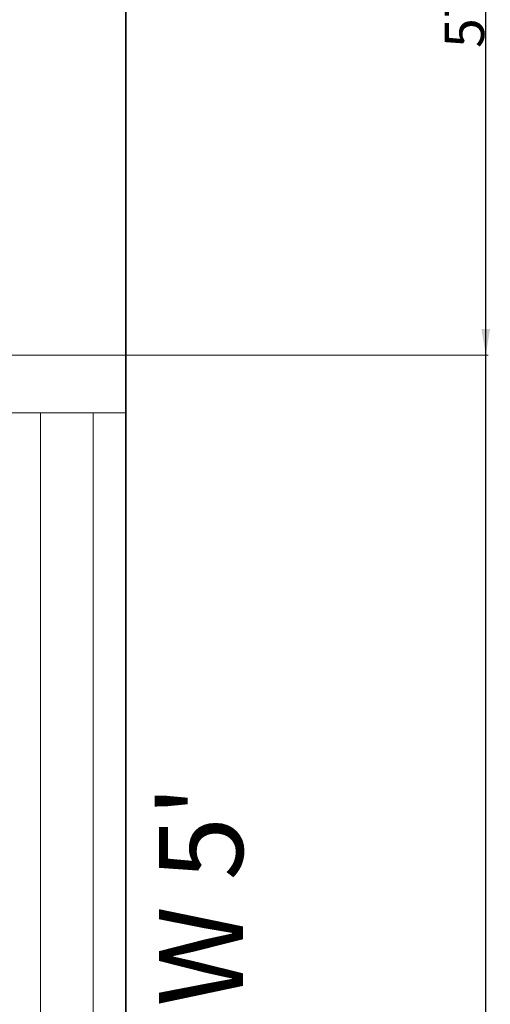
# Model space of a CAD drawing. Units: feet. Extents: x -297 to 770, y -228 to 625.
# Tile 13 of 14: x 734 to 770, y 158 to 233. Entities that reach past the tile are written whole.
import ezdxf

# ---------------------------------------------------------------- set-up
doc = ezdxf.new("R2010")
doc.units = ezdxf.units.FT
doc.header["$MEASUREMENT"] = 0
for name, color, linetype, lineweight in [('A-ANNO-DIMS', 2, 'Continuous', 18), ('A-ANNO-TEXT', 7, 'Continuous', 18), ('A-WALL', 7, 'Continuous', 35), ('windows', 30, 'Continuous', 18)]:
    doc.layers.add(name, color=color, linetype=linetype, lineweight=lineweight)
doc.styles.add('Annotative', font='arial.ttf')
doc.styles.get("Standard").update_dxf_attribs({"font": 'arial.ttf'})
doc.dimstyles.get("Standard").update_dxf_attribs({"dimtxt": 3, "dimasz": 2, "dimexe": 0.18, "dimexo": 0.0625, "dimgap": 0.09, "dimtad": 1, "dimtoh": 1, "dimdec": 1, "dimzin": 0, "dimdsep": 46, "dimlunit": 3, "dimtxsty": 'Standard', "dimcen": 0, "dimclre": 256, "dimadec": 0, "dimazin": 0, "dimtfac": 1, "dimtdec": 1, "dimtofl": 0, "dimtmove": 0, "dimatfit": 3, "dimfxl": 1, "dimtolj": 1, "dimtzin": 0, "dimlwe": -1, "dimarcsym": 0})

# ---------------------------------------------------------------- blocks, each defined once
blk = doc.blocks.new('WIN-5FT')
for p, q in [((60, 6.5), (0, 6.5)), ((60, 2.5), (0, 2.5))]:
    blk.add_line(p, q)
blk.add_lwpolyline([(60, 0), (60, 9), (0, 9), (0, 0)], close=True)
blk = doc.blocks.new('*D44')
at = {"layer": 'A-ANNO-DIMS', "transparency": 16777216}
for p, q in [((742.218, 306.963), (769.785, 306.963)), ((742.218, -200.037), (769.785, -200.037))]:
    blk.add_line(p, q, dxfattribs=at)
at = {"layer": 'A-ANNO-DIMS', "color": 0, "lineweight": -2, "transparency": 16777216}
blk.add_line((769.605, -198.037), (769.605, 304.963), dxfattribs=at)
at = {"layer": 'A-ANNO-DIMS', "color": 0, "transparency": 16777216}
for points in [[(769.272, 304.963), (769.939, 304.963), (769.605, 306.963)], [(769.272, -198.037), (769.939, -198.037), (769.605, -200.037)]]:
    blk.add_solid(points, dxfattribs=at)
at = {"layer": 'Defpoints', "color": 0, "transparency": 16777216}
for p in [(742.155, 306.963), (769.605, 306.963), (742.155, -200.037)]:
    blk.add_point(p, dxfattribs=at)
at = {"layer": 'A-ANNO-DIMS', "color": 0, "transparency": 16777216, "insert": (767.984, 53.463), "char_height": 3, "attachment_point": 5, "rotation": 90}
blk.add_mtext('\\A1;507', dxfattribs=at)
blk = doc.blocks.new('*D75')
at = {"layer": 'A-ANNO-DIMS', "transparency": 16777216}
for p, q in [((471.753, 264.961), (769.785, 264.961)), ((471.753, 207.869), (769.785, 207.869))]:
    blk.add_line(p, q, dxfattribs=at)
at = {"layer": 'A-ANNO-DIMS', "color": 0, "lineweight": -2, "transparency": 16777216}
blk.add_line((769.605, 209.869), (769.605, 262.961), dxfattribs=at)
at = {"layer": 'A-ANNO-DIMS', "color": 0, "transparency": 16777216}
for points in [[(769.272, 262.961), (769.939, 262.961), (769.605, 264.961)], [(769.272, 209.869), (769.939, 209.869), (769.605, 207.869)]]:
    blk.add_solid(points, dxfattribs=at)
at = {"layer": 'Defpoints', "color": 0, "transparency": 16777216}
for p in [(471.691, 264.961), (769.605, 264.961), (471.691, 207.869)]:
    blk.add_point(p, dxfattribs=at)
at = {"layer": 'A-ANNO-DIMS', "color": 0, "transparency": 16777216, "insert": (767.984, 236.415), "char_height": 3, "attachment_point": 5, "rotation": 90}
blk.add_mtext('\\A1;57.09', dxfattribs=at)

msp = doc.modelspace()

# ---------------------------------------------------------------- linework, layer by layer
at = {"layer": 'A-WALL'}
msp.add_line((742.155, -200.037), (742.155, 306.963), dxfattribs=at)

# ---------------------------------------------------------------- block references
at = {"layer": 'windows', "rotation": 90.00000000000003}
msp.add_blockref('WIN-5FT', (742.155, 143.463), dxfattribs=at)

# ---------------------------------------------------------------- texts
at = {"layer": 'A-ANNO-TEXT', "style": 'Annotative'}
msp.add_text("W 5'", height=6.4048, rotation=90, dxfattribs=at).set_placement((751.087, 158.16))

# ---------------------------------------------------------------- dimensions: what is measured, and where the dimension line sits
at = {"layer": 'A-ANNO-DIMS'}
for base, p1, p2, override, picture, middle in [((769.605, 306.963), (742.155, -200.037), (742.155, 306.963), {"dimdec": 0, "dimlfac": 1, "dimrnd": 0, "dimzin": 0, "dimdsep": 46, "dimlunit": 2}, '*D44', (767.984, 53.463)), ((769.605, 264.961), (471.691, 207.869), (471.691, 264.961), {"dimdec": 2, "dimlfac": 1, "dimrnd": 0, "dimzin": 0, "dimdsep": 46, "dimlunit": 2}, '*D75', (767.984, 236.415))]:
    dim = msp.add_linear_dim(base=base, p1=p1, p2=p2, angle=90, dimstyle='Standard', override=override, dxfattribs=at)
    dim.commit()
    dim.dimension.update_dxf_attribs({"geometry": picture, "text_midpoint": middle})

doc.saveas('drawing.dxf')
